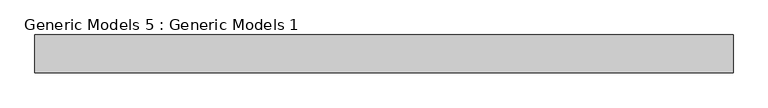
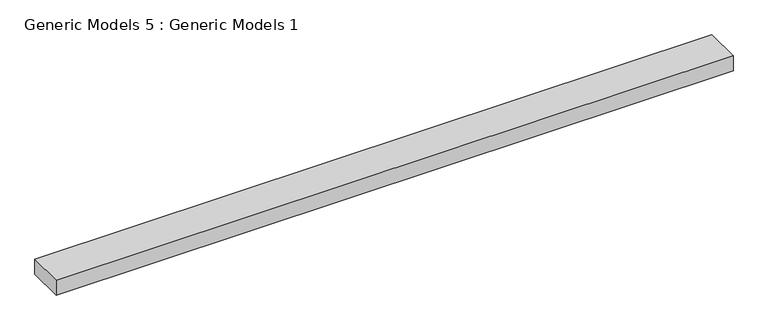
"""IFC4 building model written with IfcOpenShell, lengths in millimetres: proxy geometry, Generic Models 5 : Generic Models 1."""

from ifc_helpers import new_model, si_unit, frame, origin, place, context, project, spatial, polyline, outline, extrude, source, transform, mapped, element, save


def generic_models_5_generic_models_1_92fab196(model_context):
    return source(origin(), model_context, "Body", "SweptSolid", [
        extrude(outline(polyline([(179.4173869, -8059.5844117), (-11107.9539306, -8059.5844117), (-11107.9539306, -7449.9844117), (179.4173869, -7449.9844117), (179.4173869, -8059.5844117)])), frame((0.0, 0.0, 6137.7541096), z_axis=(0.0, 0.0, 1.0), x_axis=(1.0, 0.0, 0.0)), (0.0, 0.0, 1.0), 263.0458904),
    ])


if __name__ == "__main__":
    model = new_model("IFC4")
    model_context = context("Model", 3, world=origin())
    ifc_project = project(units=[si_unit("LENGTHUNIT", "METRE", prefix="MILLI")], contexts=[model_context])
    site = spatial("IfcSite", under=ifc_project)
    building = spatial("IfcBuilding", under=site)
    placement = place(None, origin())
    generic_models_5_generic_models_1_shape = generic_models_5_generic_models_1_92fab196(model_context)
    element("IfcBuildingElementProxy", 1, Name="Generic Models 5 : Generic Models 1", ObjectType="Generic Models 5 : Generic Models 1", at=placement, inside=building, context=model_context, shape_type="MappedRepresentation", body=[
        mapped(generic_models_5_generic_models_1_shape, transform((0.0, 0.0, 0.0), x_axis=(1.0, 0.0, 0.0), y_axis=(0.0, 1.0, 0.0), z_axis=(0.0, 0.0, 1.0))),
    ])
    save(model, "model.ifc")

# Revit data of these elements
# Element 1 (IfcBuildingElementProxy, "Generic Models 5 : Generic Models 1")
#   Materials on its faces: "Clad - White"
# Materials
#   "Clad - White": class "Wood", colour RGB 242 242 238, transparency 0, Cost = 0
